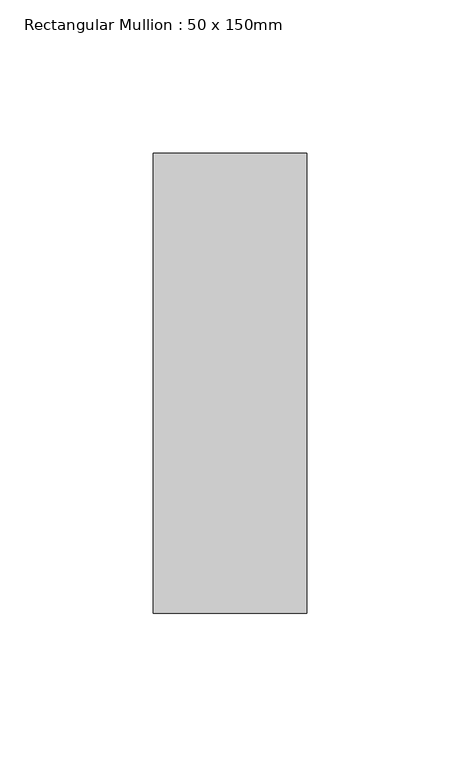
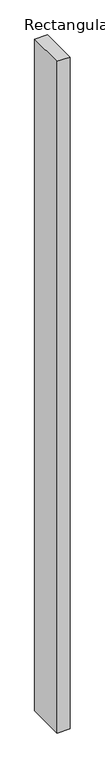
"""IFC4 building model written with IfcOpenShell, lengths in millimetres: member geometry, Rectangular Mullion : 50 x 150mm."""

from ifc_helpers import new_model, si_unit, frame, origin, place, context, project, spatial, polyline, outline, extrude, source, transform, mapped, element, save


def rectangular_mullion_50_x_150mm_0da89c4c(model_context):
    return source(origin(), model_context, "Body", "SweptSolid", [
        extrude(outline(polyline([(0.0, 75.0), (0.0, -75.0), (-50.0, -75.0), (-50.0, 75.0), (0.0, 75.0)])), frame((0.0, 0.0, -2743.2), z_axis=(0.0, 0.0, 1.0), x_axis=(1.0, 0.0, 0.0)), (0.0, 0.0, 1.0), 2743.2),
    ])


if __name__ == "__main__":
    model = new_model("IFC4")
    model_context = context("Model", 3, world=origin())
    ifc_project = project(units=[si_unit("LENGTHUNIT", "METRE", prefix="MILLI")], contexts=[model_context])
    site = spatial("IfcSite", under=ifc_project)
    building = spatial("IfcBuilding", under=site)
    placement = place(None, origin())
    rectangular_mullion_50_x_150mm_shape = rectangular_mullion_50_x_150mm_0da89c4c(model_context)
    element("IfcMember", 1, ObjectType="Rectangular Mullion : 50 x 150mm", at=placement, inside=building, context=model_context, shape_type="MappedRepresentation", body=[
        mapped(rectangular_mullion_50_x_150mm_shape, transform((0.0, 0.0, 0.0), x_axis=(1.0, 0.0, 0.0), y_axis=(0.0, 1.0, 0.0), z_axis=(0.0, 0.0, 1.0))),
    ])
    save(model, "model.ifc")

# Revit data of these elements
# Type "Rectangular Mullion : 50 x 150mm"
#   built-in parameter 1007304 = 0.492126 (stored number, unit not read)
#   built-in parameter 1007301 = 0.082021 (stored number, unit not read)
#   built-in parameter 1007300 = 0.082021 (stored number, unit not read)
# Element 1 (IfcMember, "Rectangular Mullion : 50 x 150mm")
#   Materials on its faces: "Aluminium"
# Materials
#   "Aluminium": class "Metal", colour RGB 247 247 247, transparency 0, Description = "Aluminium 6061", Cost = 0
